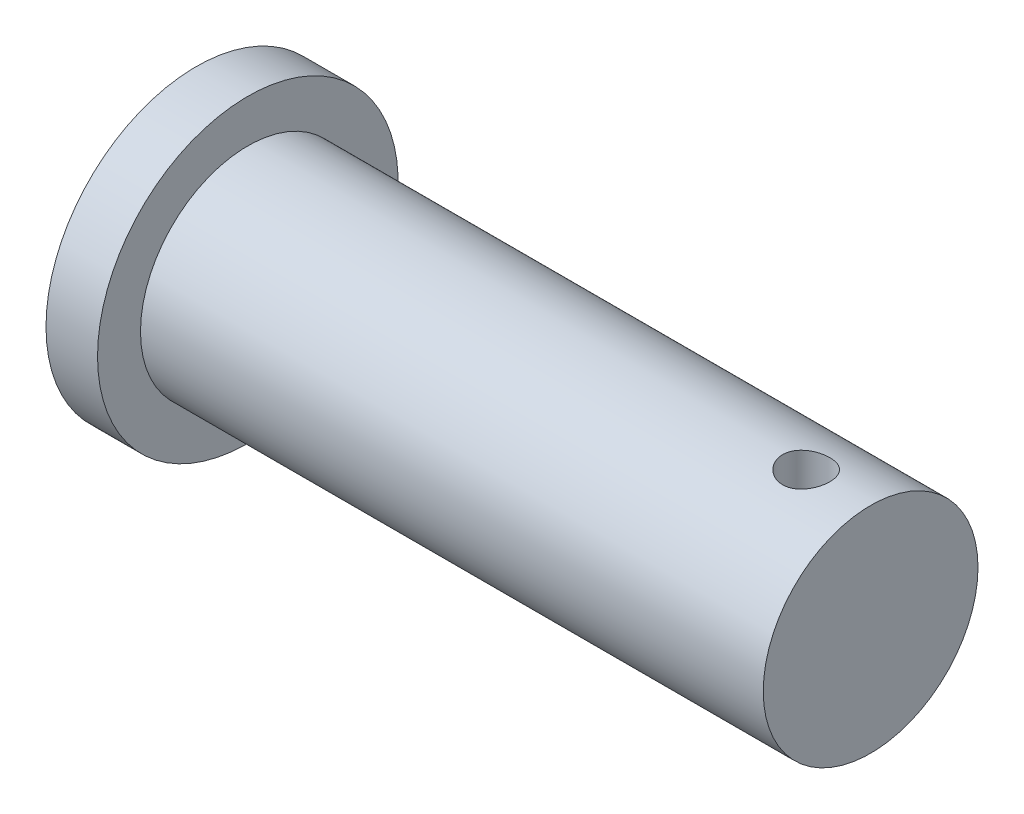
from build123d import *

# Parameters (mm, degrees)
SPLIT_PIN_HOLE_SKETCH_R = 5.486925686
SPLIT_PIN_HOLE_11_DEPTH = 30


with BuildPart() as part:
    # Pin Profile Sketch → Pin Body Revolve (revolve)
    with BuildSketch(Plane.XY, mode=Mode.PRIVATE) as pin_body_revolve_sk:
        Polygon((0, 0), (0, 25), (-145, 25), (-145, 35), (-157, 35), (-157, 0), align=None)
    revolve(pin_body_revolve_sk.sketch.rotate(Axis((-157, 0, 0), (1, 0, 0)), 90), axis=Axis((-157, 0, 0), (1, 0, 0)))

    # Split Pin Hole Sketch → Split Pin Hole Ø11 (cut, symmetric)
    with BuildSketch(Plane(origin=(0, 0, 0), x_dir=(1, 0, 0), z_dir=(0, 1, 0))):
        with Locations(Location((-15, 0, 0), (0, 0, 270))):
            Circle(SPLIT_PIN_HOLE_SKETCH_R)
    extrude(amount=SPLIT_PIN_HOLE_11_DEPTH, both=True, mode=Mode.SUBTRACT)


solid = part.part
